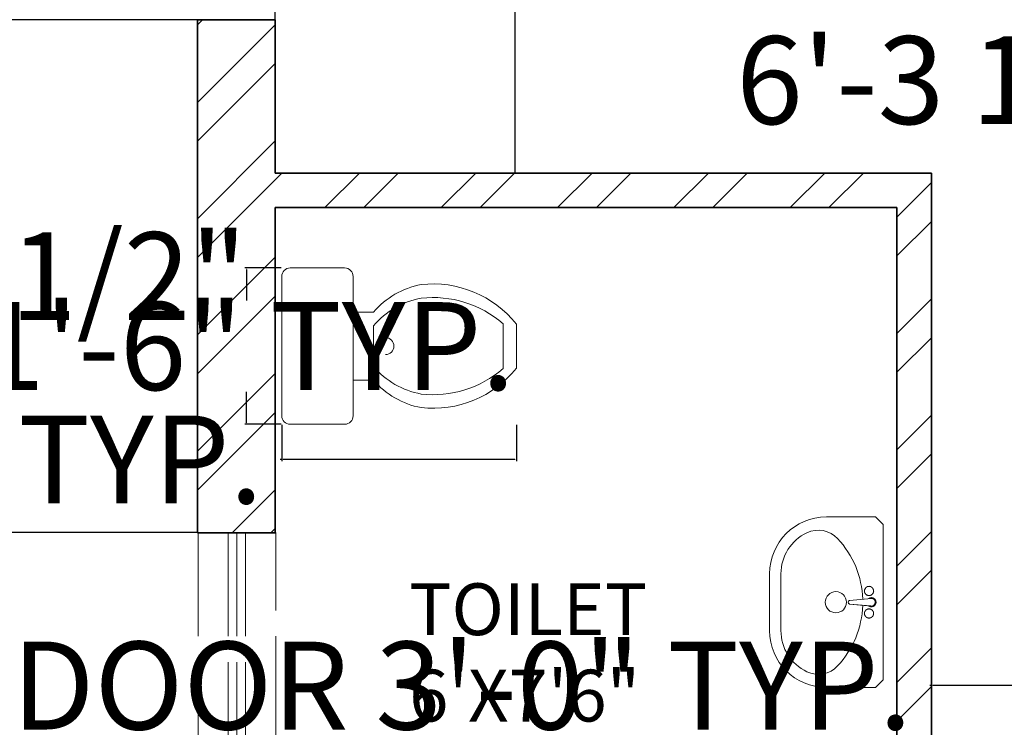
# Model space of a CAD drawing. Units: inches. Extents: x 1812 to 2791, y 2306 to 2959.
# Tile 3 of 8: x 1870 to 1984, y 2774 to 2856. Entities that reach past the tile are written whole.
import ezdxf

# ---------------------------------------------------------------- set-up
doc = ezdxf.new("R2010")
doc.units = ezdxf.units.IN
doc.linetypes.add('ACAD_ISO02W100', pattern=[15, 12, -3])
doc.layers.get('Defpoints').update_dxf_attribs({"lineweight": 50})
for name, color, linetype, lineweight in [('A-ANNO-DIMS', 2, 'Continuous', 18), ('A-AREA-IDEN', 7, 'Continuous', 18), ('A-FLOR-CASE', 8, 'Continuous', 18), ('A-FLOR-FIXT', 9, 'Continuous', 18), ('A-GLAZ-VENT', 6, 'ACAD_ISO02W100', 13), ('A-WALL-PATT', 8, 'Continuous', 13), ('WALL', 7, 'Continuous', 35)]:
    doc.layers.add(name, color=color, linetype=linetype, lineweight=lineweight)
doc.styles.get("Standard").update_dxf_attribs({"font": 'arial.ttf'})
doc.dimstyles.get("Standard").update_dxf_attribs({"dimtxt": 10.18, "dimasz": 0.18, "dimexe": 0.18, "dimexo": 0.0625, "dimgap": 0.09, "dimtad": 0, "dimtih": 1, "dimtoh": 1, "dimdec": 0, "dimzin": 0, "dimdsep": 46, "dimlunit": 3, "dimtxsty": 'Standard', "dimcen": 0.09, "dimadec": 0, "dimazin": 0, "dimtfac": 1, "dimtdec": 0, "dimtofl": 0, "dimtmove": 0, "dimatfit": 3, "dimfxl": 1, "dimtolj": 1, "dimtzin": 0, "dimarcsym": 0})

# ---------------------------------------------------------------- blocks, each defined once
blk = doc.blocks.new('A$C2AC94788')
for p, q in [((0.0250000842625013, 0.6899999873276103), (0.4350000842623559, 0.6899999873276103)), ((8.42619556e-08, 0.5049999873299384), (8.42619556e-08, 0.664999987326155)), ((0.4600000842619921, 0.664999987326155), (0.4600000842619921, 0.5049999873299384)), ((0.4350000842623559, 0.4799999873284833), (0.0250000842625013, 0.4799999873284833)), ((0.1300000842620648, 0.4799999873284833), (0.1300000842620648, 0.4199999873308116)), ((0.3300000842618829, 0.4199999873308116), (0.3300000842618829, 0.4799999873284833)), ((0.1700000842620284, 0.4199999873308116), (0.2900000842619192, 0.4199999873308116)), ((0.1640625266463758, 0.0391832446184708), (0.2959376418775719, 0.0391832446184708)), ((0.2290625266468851, 0.0391832446184708), (0.2300046331329213, 0.0391832446184708)), ((0.2309376418770626, 0.0391832446184708), (0.2299955353910263, 0.0391832446184708)), ((0.1650000842619192, -1.26747182e-08), (0.2950000842620284, -1.26747182e-08))]:
    blk.add_line(p, q)
for centre, radius, start, end in [((0.0250000842625013, 0.664999987326155), 0.025, 90, 180), ((0.4350000842623559, 0.664999987326155), 0.025, 0, 90), ((0.0250000842625013, 0.5049999873299384), 0.025, 180, 270), ((0.4350000842623559, 0.5049999873299384), 0.025, 270, 0), ((0.2874442183401697, 0.2355819240110577), 0.2424843859558644, 130.488541879527, 169.445013547103), ((0.3274442183401334, 0.2355819240110577), 0.2424843859558644, 130.488541879527, 169.445013547103), ((0.1325559501838143, 0.2355819240110577), 0.2424843859558745, 10.55498645289699, 49.51145812047296), ((0.1725559501837779, 0.2355819240110577), 0.2424843859558745, 10.55498645289699, 49.51145812047296), ((0.2300000842624286, 0.3849999873273191), 0.025, 180, 0), ((0.3600593119572294, 0.2447691737834247), 0.3129857136460789, 173.5368801771597, 231.4482773914608), ((0.4000593119571932, 0.2447691737834248), 0.3129857136460972, 173.5368801771598, 221.0603827222079), ((0.0999408565667182, 0.2447691737834248), 0.3129857136460789, 308.5517226085392, 6.463119822840183), ((0.0599408565667545, 0.2447691737834248), 0.3129857136460896, 318.9396172777922, 6.463119822840183)]:
    blk.add_arc(centre, radius, start, end)
blk = doc.blocks.new('s_46')
at = {"ltscale": 600}
h = blk.add_hatch(color=256, dxfattribs=at)
edge = h.paths.add_edge_path()
edge.add_line((13.45184378023259, 62.04360352296498), (14.15927104179718, 54.09782096462731))
edge.add_ellipse((4.212458010588306, 52.31250418393756), major_axis=(-10.10576298371302, 2.5e-15), ratio=1, start_angle=540, end_angle=550.1754626554052, ccw=False)
edge.add_arc((4.212458010588306, 52.31250418393756), 10.10576298371302, 270, 360, ccw=False)
edge.add_line((4.212458010588306, 42.20674120020703), (4.212458010588306, 41.28018079043977))
edge.add_line((4.212458010588306, 41.28018079040339), (11.85106942148559, 41.28018079040339))
edge.add_arc((4.212458010588306, 52.31250418393756), 13.41866400745597, 664.6981342835142, 766.4847699121552)
h.paths.add_polyline_path([(4.212458010588306, 41.28018079040339), (-3.426153400272596, 41.28018079040339, 0.152566653256377), (4.212458010588306, 38.8938401764608)])
h.paths.add_polyline_path([(11.85106942144921, 41.28018079040339), (4.212458010588306, 41.28018079040339), (4.212458010588306, 38.8938401764608, 0.1525666532563772)])
h.paths.add_polyline_path([(-5.734355020395014, 54.09782096461277), (-5.026927758881356, 62.04360352296498, 0.4758332592079194), (-3.426153400272596, 41.28018079040339), (4.212458010588306, 41.28018079040339), (4.212458010588306, 42.20674120020703, -0.4672400657637396)])
for p, q in [((-5.893304973142221, 52.31250418385025), (-0.714987907151226, 110.4750654234667)), ((-5.893304973142221, 52.31250418385025), (-0.714987907151226, 110.4750654234667)), ((9.139903928502463, 110.475065423554), (14.15927104174625, 54.09782096461277)), ((14.31822099431883, 52.31250418385025), (9.139903928502463, 110.475065423554)), ((14.15927104174625, 54.09782096461277), (14.31822099431883, 52.31250418385025))]:
    blk.add_line(p, q, dxfattribs=at)
blk.add_lwpolyline([(-220.7875419894117, 171.2801807903452, -0.4142135623730951), (-70.7875419894117, 321.2801807903452), (79.2124580105883, 321.2801807904325, -0.4142135623730951), (229.2124580105883, 171.2801807904325), (229.2124580105883, 41.28018079040339), (209.2124580107047, 21.2801807904325), (-200.7875419893535, 21.28018079034518), (-220.7875419894117, 41.28018079040339)], format="xyb", close=True, dxfattribs=at)
blk.add_lwpolyline([(12.26164246437838, 75.41187665969483, 0.1816379869150311), (172.1859176590806, 141.5383421540609, 0.3263505073803008), (187.6570333366981, 222.6589125997853, 0.2898144196813102), (79.21245801076293, 291.2801807904325), (-70.78754198923707, 291.2801807903452, 0.2898144196813102), (-179.2321173155214, 222.658912599698, 0.3263505073803008), (-163.7610016377293, 141.5383421540609, 0.1816379869150315), (-3.836726442852523, 75.41187665960751)], format="xyb", dxfattribs=at)
for points in [[(-16.83803374727722, 67.43055756771354), (-17.02338931558188, 67.50428807432763), (-17.22058725368697, 67.56961317334208), (-17.42189012444578, 67.6347039079701), (-17.61956049106084, 67.70773132116301), (-17.80586091603618, 67.79686645595939), (-17.97305396257434, 67.91028035557245), (-18.11578784312587, 68.05326030802098), (-18.23825336818117, 68.21955858168076), (-18.34702699835179, 68.40004368982045), (-18.44868519355077, 68.58558414605795), (-18.54980441438965, 68.76704846357461), (-18.65696112113073, 68.9353051558137), (-18.77673177386168, 69.08122273621848), (-18.91569283319404, 69.19566971814493), (-19.07841429975815, 69.27267628890695), (-19.26144033775199, 69.31891933156292), (-19.45930865121772, 69.34423740339116), (-19.66655694507062, 69.35846906132065), (-19.87772292352747, 69.37145286262967), (-20.08734429115429, 69.39302736415993), (-20.2899587523425, 69.43303112310241), (-20.48010401183274, 69.50130269664805), (-20.65391131333308, 69.60429419830325), (-20.81388605764368, 69.73491196823306), (-20.96412718523061, 69.8826759030926), (-21.10873363655992, 70.03710589953698), (-21.25180435174844, 70.18772185422131), (-21.39743827126222, 70.3240436638007), (-21.54973433539272, 70.43559122501756), (-21.71279148443137, 70.5118844343524), (-21.88955151231494, 70.54600451889564), (-22.07832762773614, 70.54527802669325), (-22.27627589285839, 70.52059283622657), (-22.4805523698451, 70.48283682571491), (-22.68831312085968, 70.44289787355228), (-22.89671420806553, 70.41166385821998), (-23.10291169380071, 70.40002265802468), (-23.30406164005399, 70.41886215136037), (-23.49802141042892, 70.4753938675276), (-23.68545357254334, 70.56212393892929), (-23.86772199510597, 70.66788214896224), (-24.04619054717477, 70.78149828102323), (-24.22222309763311, 70.89180211850908), (-24.39718351518968, 70.98762344472925), (-24.57243566872785, 71.05779204316786), (-24.74934342730558, 71.09113769704709), (-24.92903553397628, 71.08022740500746), (-25.11170022917213, 71.03257702605333), (-25.2972906283685, 70.95943963443278), (-25.48575984616764, 70.8720683044812), (-25.67706099752104, 70.7817161102721), (-25.87114719772944, 70.69963612605352), (-26.0679715613951, 70.63708142607356), (-26.26748720381875, 70.60530508466763), (-26.46941223740578, 70.61182491958607), (-26.67252476507565, 70.64921772302478), (-26.87536788737634, 70.70632503094384), (-27.07648470485583, 70.77198837930337), (-27.27441831788747, 70.8350493038015), (-27.46771182701923, 70.88434934031102), (-27.6549083327991, 70.90873002487933), (-27.83455093560042, 70.8970328932919), (-28.00620139669627, 70.84190539614065), (-28.17349611973623, 70.75121864315588), (-28.34109016874572, 70.63664965887438), (-28.51363860827405, 70.50987546765828), (-28.69579650234664, 70.38257309404435), (-28.89221891516354, 70.26641956248204), (-29.10756091127405, 70.17309189750813), (-29.3464775547036, 70.11426712348475), (-29.61160253512208, 70.0940409177856), (-29.89748404390411, 70.0861835690448), (-30.19664889771957, 70.05688401864609), (-30.50162391323829, 69.9723312081478), (-30.80493590747938, 69.79871407902101), (-31.09911169676343, 69.50222157256212), (-31.37667809793493, 69.0490426304168), (-31.63016192783834, 68.40536619405611), (-32.32050594605971, 68.4500712644367), (-32.84873653826071, 68.3918758847285), (-33.24226493795868, 68.25193804170704), (-33.52850237919483, 68.0514157223224), (-33.73486009566113, 67.8114669136994), (-33.88874932087492, 67.5532496026135), (-34.01758128887741, 67.29792177610216), (-34.14876723336056, 67.06664142102818), (-34.30371923936764, 66.87550954936887), (-34.47985279804561, 66.72039927294827), (-34.66858425136889, 66.59212672835565), (-34.86132994201034, 66.48150805244222), (-35.04950621211901, 66.37935938188457), (-35.22452940384392, 66.27649685335928), (-35.37781585985795, 66.16373660371755), (-35.50078192248475, 66.03189476963598), (-35.58785390376579, 65.87432967920904), (-35.64549799636007, 65.69456842611542), (-35.68319036299363, 65.49868029527715), (-35.7104071660433, 65.2927345718781), (-35.73662456823513, 65.08280054092756), (-35.77131873212056, 64.87494748734753), (-35.82396582007641, 64.67524469623459), (-35.90404199482873, 64.48976145259803), (-36.01774371694773, 64.3227640100813), (-36.15814863995183, 64.17130649695173), (-36.31505471485434, 64.0306400101108), (-36.47825989319244, 63.89601564637269), (-36.63756212632871, 63.76268450255157), (-36.78275936545106, 63.62589767554891), (-36.90364956192207, 63.48090626226621), (-36.99003066710429, 63.32296135951764), (-37.03518227743916, 63.14869254492805), (-37.04631056915969, 62.96024331927765), (-37.03410336375237, 62.7611356638954), (-37.00924848217983, 62.55489156045951), (-36.98243374592858, 62.34503299021162), (-36.96434697631048, 62.13508193491725), (-36.96567599463743, 61.92856037581805), (-36.99710862222128, 61.72899029450491), (-37.06570762058254, 61.53896291530691), (-37.16403551277472, 61.35734643402975), (-37.28102976223454, 61.18207828939194), (-37.40562783187488, 61.0110959201993), (-37.52676718513249, 60.84233676508302), (-37.63338528544409, 60.67373826284892), (-37.7144195958972, 60.50323785204091), (-37.75880757992855, 60.32877297155209), (-37.75920177751686, 60.14875038337777), (-37.72311503690435, 59.96345414296957), (-37.66177528270055, 59.77363762940512), (-37.58641044021351, 59.58005422132555), (-37.5082484340528, 59.38345729780849), (-37.43851718935184, 59.18460023758234), (-37.38844463089481, 58.98423641963745), (-37.36925868364051, 58.78311922278953), (-37.38844463089481, 58.58200202594161), (-37.43851718935184, 58.38163820799673), (-37.5082484340528, 58.18278114777058), (-37.58641044021351, 57.98618422425352), (-37.66177528287517, 57.79260081626126), (-37.72311503690435, 57.6027843026095), (-37.75920177751686, 57.4174880622013), (-37.75880757992855, 57.23746547402697), (-37.7144195958972, 57.06300059353816), (-37.63338528544409, 56.89250018273014), (-37.52676718530711, 56.72390168049606), (-37.40562783187488, 56.55514252537978), (-37.28102976223454, 56.38416015618713), (-37.16403551277472, 56.20889201154932), (-37.06570762058254, 56.02727553035947), (-36.99710862222128, 55.83724815107416), (-36.96567599463743, 55.63767806976102), (-36.96434697631048, 55.43115651066182), (-36.98243374592858, 55.22120545536745), (-37.00924848217983, 55.01134688520687), (-37.03410336375237, 54.80510278168367), (-37.04631056933431, 54.60599512638873), (-37.03518227743916, 54.41754590065102), (-36.99003066710429, 54.24327708606142), (-36.90364956192207, 54.08533218331285), (-36.78275936545106, 53.94034077003016), (-36.63756212632871, 53.80355394302751), (-36.47825989319244, 53.67022279920639), (-36.31505471502896, 53.53559843546827), (-36.15814863995183, 53.39493194862734), (-36.01774371712236, 53.24347443549777), (-35.90404199482873, 53.07647699298104), (-35.82396582007641, 52.89099374934449), (-35.77131873212056, 52.69129095823155), (-35.73662456823513, 52.48343790465151), (-35.71040716621792, 52.27350387370098), (-35.68319036299363, 52.06755815021461), (-35.64549799653469, 51.87167001946363), (-35.58785390376579, 51.69190876637003), (-35.50078192248475, 51.53434367594309), (-35.3778353385278, 51.40284301002975), (-35.22468523163116, 51.29247093791491), (-35.05003213009331, 51.19609060572111), (-34.86257656256203, 51.10656515930895), (-34.67101905716118, 51.01675774488831), (-34.48406014236389, 50.91953150840708), (-34.31040034646867, 50.80774959607516), (-34.15874019777402, 50.67427515375311), (-34.03505195630714, 50.51453334218241), (-33.93439480883535, 50.3341973797942), (-33.84909967368003, 50.14150249981321), (-33.77149746881332, 49.94468393520219), (-33.69391911290586, 49.75197691909852), (-33.60869552427903, 49.57161668455228), (-33.50815762107959, 49.41183846470085), (-33.38463632145431, 49.28087749250699), (-33.23284944484476, 49.18408373402781), (-33.05706241185544, 49.11526608630083), (-32.86392754490953, 49.06534817945794), (-32.66009716555709, 49.02525364354369), (-32.45222359569743, 48.98590610860265), (-32.24695915722987, 48.93822920459206), (-32.05095617187908, 48.87314656155649), (-31.870866961719, 48.78158180962782), (-31.71133844077122, 48.65761859554914), (-31.5689958925941, 48.50798063381808), (-31.43845919286832, 48.34255165536887), (-31.31434821744915, 48.17121539139771), (-31.19128284219187, 48.00385557310073), (-31.06388294277713, 47.85035593167413), (-30.92676839523483, 47.72060019822674), (-30.77455907507101, 47.62447210386745), (-30.60346923320321, 47.56846716045401), (-30.41609062027419, 47.54552800310193), (-30.21660936163971, 47.54520904741366), (-30.00921158283018, 47.55706470907898), (-29.79808340937598, 47.570649403875), (-29.58741096680751, 47.57551754757878), (-29.38138038065517, 47.56122355579281), (-29.18417777627474, 47.51732184420689), (-28.99883273948217, 47.43692629240103), (-28.8237486963626, 47.32738863455597), (-28.65617253311211, 47.19962006882997), (-28.49335113610141, 47.06453179311938), (-28.33253139152657, 46.9330350055825), (-28.1709601857583, 46.81604090429027), (-28.00588440499268, 46.72446068713907), (-27.83455093577504, 46.66920555219985), (-27.6549083327991, 46.65750842061243), (-27.46771182701923, 46.68188910518074), (-27.27441831788747, 46.73118914177758), (-27.07648470485583, 46.7942500662757), (-26.87536788755096, 46.85991341454792), (-26.67252476525027, 46.91702072246698), (-26.4694122375804, 46.95441352590569), (-26.26748720399337, 46.96093336082412), (-26.06797156156972, 46.9291570194182), (-25.87114719772944, 46.86660231943824), (-25.67706099769566, 46.78452233530697), (-25.48575984616764, 46.69417014101054), (-25.2972906283685, 46.60679881105898), (-25.11170022934675, 46.53366141943843), (-24.92903553397628, 46.4860110404843), (-24.74934342730558, 46.47510074844467), (-24.57243566890247, 46.50844640232389), (-24.39718351536431, 46.57861500076251), (-24.22222309780773, 46.67443632698268), (-24.0461905473494, 46.78474016446853), (-23.86772199528059, 46.89835629652953), (-23.68545357254334, 47.00411450656247), (-23.49802141060354, 47.09084457796416), (-23.30406164022861, 47.14737629413138), (-23.10291169380071, 47.16621578746708), (-22.89671420806553, 47.15457458727178), (-22.68831312085968, 47.12334057193948), (-22.4805523698451, 47.08340161977685), (-22.27627589285839, 47.04564560926519), (-22.07832762791077, 47.02096041871118), (-21.88955151248956, 47.02023392650881), (-21.71279148443137, 47.05435401113937), (-21.54973433539272, 47.1306472204742), (-21.39743827126222, 47.24219478160375), (-21.25180435174844, 47.37851659118314), (-21.10873363655992, 47.52913254586746), (-20.96412718540523, 47.68356254231185), (-20.81388605764368, 47.83132647717138), (-20.65391131333308, 47.9619442471012), (-20.48010401200736, 48.0649357488437), (-20.28995875251712, 48.13320732230204), (-20.08734429115429, 48.17321108133183), (-19.87772292352747, 48.1947855828621), (-19.66655694507062, 48.2077693840838), (-19.45930865139235, 48.2220010421006), (-19.26144033775199, 48.24731911384152), (-19.07841429993277, 48.29356215667212), (-18.91569283319404, 48.37056872743414), (-18.77673177403631, 48.48501570936059), (-18.65696112113073, 48.63093328976538), (-18.54980441456428, 48.79918998200446), (-18.44868519372539, 48.98065429960843), (-18.34702699835179, 49.16619475575862), (-18.2382533683558, 49.34667986398562), (-18.11578784312587, 49.5129781376454), (-17.97305396274896, 49.6559580900066), (-17.8058609162108, 49.76937198961969), (-17.61956049106084, 49.85850712450337), (-17.4218901246204, 49.93153453769628), (-17.22058725368697, 49.996625272237), (-17.02338931558188, 50.06195037133875), (-16.83803374727722, 50.13568087795284), (-16.67225798609434, 50.22598783511785), (-16.53379946883069, 50.34104228604701), (-16.42766593385022, 50.48645191569812), (-16.34794632298872, 50.65757097714231), (-16.28599987912457, 50.84719036528259), (-16.23318584513618, 51.04810097528389), (-16.18086346407654, 51.25309370196191), (-16.12039197882404, 51.45495944039431), (-16.04313063243171, 51.64648908557137), (-15.94043866742868, 51.82047353248345), (-15.8067031877581, 51.97190354572376), (-15.64842273970134, 52.10456936812261), (-15.47512373042991, 52.22446111202589), (-15.29633256676607, 52.33756888969219), (-15.12157565605594, 52.44988281364204), (-14.96037940529641, 52.567392996134), (-14.82227022130973, 52.69608954960131), (-14.71677451161667, 52.84196258638985), (-14.6501372611965, 53.00919824198354), (-14.61547776852967, 53.19476674450561), (-14.60263391025364, 53.3938343450427), (-14.60144356318051, 53.60156729485606), (-14.60174460412236, 53.81313184503233), (-14.59337490954203, 54.02369424700736), (-14.566172356077, 54.22842075169319), (-14.50997482053935, 54.42247761052567), (-14.41809999983525, 54.6024088327249), (-14.29778487142175, 54.77026946117985), (-14.1597462335485, 54.92949229647638), (-14.01470088359201, 55.08351013963693), (-13.87336561962729, 55.23575579150929), (-13.7464572393801, 55.38966205302859), (-13.64469254092546, 55.54866172495531), (-13.5787883218145, 55.71618760822457), (-13.55583441938506, 55.89474125843844), (-13.56841282837558, 56.08309925056528), (-13.60547858278733, 56.27910691397847), (-13.65598671662155, 56.48060957840062), (-13.70889226370491, 56.68545257346704), (-13.7531502583879, 56.89148122872575), (-13.7777157346718, 57.09654087381204), (-13.77154372638324, 57.29847683827393), (-13.72730239736847, 57.49560352915432), (-13.65251243085367, 57.68811166286468), (-13.55840763938613, 57.8766610333987), (-13.45622183586238, 58.06191143448813), (-13.35718883317895, 58.24452266012667), (-13.27254244388314, 58.42515450413339), (-13.2135164810461, 58.60446676041465), (-13.19134475721512, 58.78311922278953), (-13.2135164810461, 58.96177168516442), (-13.27254244388314, 59.14108394144569), (-13.35718883317895, 59.3217157854524), (-13.45622183586238, 59.50432701109093), (-13.55840763938613, 59.68957741218037), (-13.65251243085367, 59.87812678271438), (-13.72730239736847, 60.07063491642475), (-13.77154372638324, 60.26776160730515), (-13.7777157346718, 60.46969757176703), (-13.7531502583879, 60.67475721685332), (-13.70889226370491, 60.88078587211203), (-13.65598671662155, 61.08562886717845), (-13.60547858278733, 61.2871315316006), (-13.56841282837558, 61.48313919501379), (-13.55583441938506, 61.67149718714063), (-13.5787883218145, 61.8500508373545), (-13.64469254092546, 62.01757672062377), (-13.7464572393801, 62.17657639255048), (-13.87336561962729, 62.33048265406978), (-14.01470088359201, 62.48272830594214), (-14.15974623337388, 62.63674614910269), (-14.29778487142175, 62.79596898448653), (-14.41809999983525, 62.96382961285416), (-14.50997482053935, 63.14376083514071), (-14.566172356077, 63.33781769388588), (-14.59337490936741, 63.5425441985717), (-14.60174460412236, 63.75310660054674), (-14.60144356318051, 63.96467115081032), (-14.60263391025364, 64.17240410053635), (-14.61547776835505, 64.37147170116077), (-14.65013726102188, 64.55704020359553), (-14.71677451144205, 64.7242758591892), (-14.82227022130973, 64.87014889597776), (-14.96037940529641, 64.99884544944507), (-15.12157565605594, 65.11635563193704), (-15.29633256676607, 65.22866955588688), (-15.47512373042991, 65.3417773336405), (-15.64842273970134, 65.46166907745646), (-15.8067031877581, 65.59433489985531), (-15.94043866742868, 65.74576491309563), (-16.04313063225709, 65.9197493600077), (-16.12039197882404, 66.11127900527208), (-16.18086346407654, 66.31314474370447), (-16.23318584513618, 66.5181374703825), (-16.28599987912457, 66.71904808029649), (-16.34794632298872, 66.90866746843676), (-16.42766593385022, 67.07978652988095), (-16.53379946883069, 67.22519615953206), (-16.67225798609434, 67.34025061046123)], [(22.08090273779817, 61.08562886709115), (22.03039460413856, 61.2871315315133), (21.99332884972682, 61.48313919501379), (21.9807504407363, 61.67149718705331), (22.00370434316574, 61.85005083726719), (22.06960856210208, 62.01757672053645), (22.17137326073134, 62.17657639246318), (22.29828164080391, 62.33048265398247), (22.43961690476863, 62.48272830585483), (22.58466225472512, 62.63674614901538), (22.72270089277299, 62.79596898439923), (22.84301602118649, 62.96382961276686), (22.93489084189059, 63.1437608350534), (22.99108837742824, 63.33781769379857), (23.01829093071865, 63.5425441985717), (23.0266606254736, 63.75310660045943), (23.02635958453175, 63.96467115072301), (23.02754993160488, 64.17240410053635), (23.04039378970629, 64.37147170107346), (23.07505328237312, 64.55704020350822), (23.14169053279329, 64.72427585910191), (23.24718624266097, 64.87014889589045), (23.38529542664764, 64.99884544935776), (23.54649167740717, 65.11635563193704), (23.7212485881173, 65.22866955579956), (23.90003975178115, 65.34177733355318), (24.07333876105258, 65.46166907736915), (24.23161920910934, 65.594334899768), (24.36535468877992, 65.74576491300832), (24.46804665360833, 65.9197493600077), (24.54530800017528, 66.11127900518477), (24.60577948542777, 66.31314474361714), (24.65810186648742, 66.51813747029519), (24.71091590047581, 66.71904808020918), (24.77286234433996, 66.90866746834945), (24.85258195520146, 67.07978652979364), (24.95871549018193, 67.22519615953206), (25.09717400744558, 67.34025061046123), (25.26294976862846, 67.43055756771354), (25.44830533693312, 67.50428807432763), (25.64550327503821, 67.56961317334208), (25.84680614579702, 67.6347039079701), (26.04447651241208, 67.70773132116301), (26.23077693756204, 67.79686645595939), (26.3979699841002, 67.91028035557245), (26.54070386447711, 68.05326030802098), (26.66316938970704, 68.21955858168076), (26.77194301970303, 68.40004368982045), (26.87360121507663, 68.58558414605795), (26.97472043591552, 68.76704846357461), (27.08187714248197, 68.9353051558137), (27.20164779538754, 69.08122273621848), (27.34060885454528, 69.19566971814493), (27.50333032128401, 69.27267628890695), (27.68635635910323, 69.31891933165025), (27.88422467274358, 69.34423740347847), (28.09147296642186, 69.35846906140794), (28.30263894487871, 69.37145286262967), (28.51226031250553, 69.39302736424725), (28.71487477386836, 69.43303112318972), (28.90502003318398, 69.50130269673537), (29.07882733468432, 69.60429419839056), (29.23880207899492, 69.73491196832038), (29.38904320658185, 69.88267590317992), (29.53364965791116, 70.0371058996243), (29.67672037309967, 70.18772185430862), (29.82235429261346, 70.324043663888), (29.97465035674395, 70.43559122501756), (30.1377075057826, 70.51188443443971), (30.31446753366618, 70.54600451898295), (30.50324364908738, 70.54527802678058), (30.70119191420963, 70.52059283622657), (30.90546839119634, 70.48283682571491), (31.11322914221091, 70.4428978736396), (31.32163022941677, 70.41166385830729), (31.52782771515195, 70.400022658112), (31.72897766157985, 70.41886215144768), (31.92293743178016, 70.4753938675276), (32.11036959389458, 70.56212393892929), (32.29263801663183, 70.66788214896224), (32.47110656870063, 70.78149828102323), (32.64713911898434, 70.89180211850908), (32.82209953654092, 70.98762344481656), (32.99735169025371, 71.05779204316786), (33.17425944865681, 71.09113769704709), (33.35395155532751, 71.08022740500746), (33.53661625069799, 71.03257702605333), (33.72220664971974, 70.9594396345201), (33.91067586751888, 70.8720683044812), (34.1019770190469, 70.7817161102721), (34.29606321908068, 70.69963612605352), (34.49288758292096, 70.63708142616088), (34.69240322534461, 70.60530508466763), (34.89432825893164, 70.61182491958607), (35.09744078660151, 70.64921772302478), (35.3002839089022, 70.70632503103116), (35.50140072620707, 70.77198837930337), (35.6993343392387, 70.8350493038015), (35.89262784837047, 70.88434934039833), (36.07982435415034, 70.90873002487933), (36.25946695695166, 70.8970328932919), (36.43111741804751, 70.84190539614065), (36.59841214108747, 70.75121864315588), (36.76600619009696, 70.63664965887438), (36.93855462962529, 70.50987546765828), (37.12071252369788, 70.38257309404435), (37.3171349366894, 70.26641956248204), (37.53247693262529, 70.17309189750813), (37.77139357605483, 70.11426712348475), (38.03651855647331, 70.0940409177856), (38.32240006525535, 70.0861835690448), (38.62156491907081, 70.05688401864609), (38.92653993476415, 69.9723312081478), (39.22985192883061, 69.79871407893368), (39.52402771811467, 69.50222157256212), (39.80159411928616, 69.0490426304168), (40.05507794918957, 68.4053661939688), (40.74542196741094, 68.4500712644367), (41.27365255961194, 68.3918758846412), (41.66718095948453, 68.25193804161972), (41.95341840054607, 68.0514157223224), (42.15977611701236, 67.8114669136121), (42.31366534240078, 67.5532496025262), (42.44249731022864, 67.29792177601485), (42.57368325471179, 67.06664142094087), (42.72863526071887, 66.87550954936887), (42.90476881939684, 66.72039927286096), (43.09350027272012, 66.59212672826834), (43.28624596336157, 66.48150805235491), (43.47442223347025, 66.37935938179726), (43.64944542536977, 66.27649685335928), (43.80273188138381, 66.16373660371755), (43.92569794383598, 66.03189476963598), (44.01276992511703, 65.87432967912173), (44.0704140177113, 65.69456842602813), (44.10810638434486, 65.49868029527715), (44.13532318739453, 65.2927345718781), (44.16154058958636, 65.08280054084025), (44.19623475347179, 64.87494748726021), (44.24888184142765, 64.67524469614727), (44.32895801617997, 64.48976145251072), (44.44265973829897, 64.32276400999397), (44.58306466130307, 64.17130649695173), (44.73997073620558, 64.03064001002348), (44.90317591454368, 63.89601564628538), (45.06247814767994, 63.76268450246425), (45.20767538680229, 63.6258976754616), (45.3285655832733, 63.4809062621789), (45.41494668845553, 63.32296135943034), (45.46009829879039, 63.14869254484074), (45.47122659051092, 62.96024331919034), (45.45901938492898, 62.76113566380809), (45.43416450353106, 62.5548915603722), (45.40734976727981, 62.34503299021162), (45.38926299766171, 62.13508193482994), (45.39059201598866, 61.92856037573074), (45.42202464357251, 61.7289902944176), (45.49062364193377, 61.53896291521959), (45.58895153412595, 61.35734643394243), (45.70594578341115, 61.18207828939194), (45.83054385322611, 61.01109592011198), (45.95168320648371, 60.84233676508302), (46.05830130679533, 60.67373826276162), (46.13933561724843, 60.50323785204091), (46.18372360127978, 60.32877297146479), (46.1841177988681, 60.14875038329046), (46.14803105825558, 59.96345414296957), (46.08669130405178, 59.77363762931782), (46.01132646156474, 59.58005422123824), (45.93316445540404, 59.38345729772118), (45.86343321070308, 59.18460023749503), (45.81336065224604, 58.98423641955014), (45.79417470499175, 58.78311922270222), (45.81336065224604, 58.58200202585431), (45.86343321070308, 58.38163820790942), (45.93316445540404, 58.18278114777058), (46.01132646156474, 57.98618422416621), (46.08669130405178, 57.79260081617394), (46.14803105808095, 57.6027843025222), (46.1841177988681, 57.4174880622013), (46.18372360127978, 57.23746547393966), (46.13933561724843, 57.06300059345085), (46.05830130679533, 56.89250018273014), (45.95168320648371, 56.72390168040874), (45.83054385322611, 56.55514252529247), (45.70594578341115, 56.38416015609982), (45.58895153412595, 56.20889201154932), (45.49062364193377, 56.02727553027216), (45.42202464339789, 55.83724815107416), (45.39059201598866, 55.63767806976102), (45.38926299766171, 55.43115651066182), (45.40734976727981, 55.22120545528014), (45.43416450335644, 55.01134688511957), (45.45901938492898, 54.80510278159636), (45.47122659051092, 54.60599512630142), (45.46009829879039, 54.41754590056371), (45.41494668845553, 54.24327708597411), (45.32856558309868, 54.08533218322554), (45.20767538662767, 53.94034076994285), (45.06247814750532, 53.8035539429402), (44.90317591454368, 53.67022279920639), (44.73997073620558, 53.53559843538096), (44.58306466130307, 53.39493194854004), (44.44265973829897, 53.24347443541046), (44.32895801617997, 53.07647699298104), (44.24888184125302, 52.89099374934449), (44.19623475329717, 52.69129095823155), (44.16154058958636, 52.48343790465151), (44.13532318739453, 52.27350387361366), (44.10810638434486, 52.06755815021461), (44.0704140177113, 51.87167001946363), (44.01276992511703, 51.69190876628272), (43.92569794366136, 51.53434367585578), (43.80275135970442, 51.40284301002975), (43.64960125280776, 51.29247093791491), (43.47494815144455, 51.1960906056338), (43.28749258373863, 51.10656515922165), (43.09593507851241, 51.01675774480099), (42.90897616371512, 50.91953150840708), (42.73531636764528, 50.80774959598784), (42.58365621895063, 50.67427515375311), (42.45996797765838, 50.51453334218241), (42.35931083018658, 50.3341973797942), (42.27401569485664, 50.14150249981321), (42.19641349016455, 49.94468393520219), (42.1188351342571, 49.75197691909852), (42.03361154545564, 49.57161668455228), (41.9330736422562, 49.41183846461354), (41.80955234280554, 49.28087749250699), (41.65776546602137, 49.1840837339405), (41.48197843320668, 49.11526608630083), (41.28884356608614, 49.06534817945794), (41.0850131867337, 49.02525364354369), (40.87713961687405, 48.98590610851534), (40.67187517840648, 48.93822920459206), (40.47587219323031, 48.87314656155649), (40.29578298289561, 48.78158180962782), (40.13625446194782, 48.65761859554914), (39.99391191377072, 48.50798063373076), (39.86337521404493, 48.34255165528157), (39.73926423862577, 48.17121539139771), (39.61619886336848, 48.00385557310073), (39.48879896395374, 47.85035593167413), (39.35168441641144, 47.72060019813944), (39.19947509624762, 47.62447210378013), (39.02838525455445, 47.56846716045401), (38.8410066414508, 47.54552800310193), (38.64152538281633, 47.54520904732635), (38.43412760400679, 47.55706470907898), (38.22299943072721, 47.570649403875), (38.01232698798413, 47.57551754757878), (37.80629640183179, 47.56122355579281), (37.60909379745135, 47.51732184420689), (37.42374876065878, 47.43692629240103), (37.24866471753922, 47.32738863455597), (37.08108855428873, 47.19962006882997), (36.91826715727803, 47.06453179311938), (36.75744741270319, 46.9330350056698), (36.59587620693492, 46.81604090429027), (36.4308004261693, 46.72446068713907), (36.25946695695166, 46.66920555228716), (36.07982435397571, 46.65750842061243), (35.89262784837047, 46.68188910518074), (35.6993343392387, 46.73118914177758), (35.50140072620707, 46.7942500662757), (35.30028390872758, 46.85991341454792), (35.09744078642689, 46.91702072246698), (34.89432825875701, 46.954413525993), (34.69240322516998, 46.96093336082412), (34.49288758274633, 46.9291570194182), (34.29606321908068, 46.86660231943824), (34.10197701887228, 46.78452233530697), (33.91067586734425, 46.69417014109785), (33.72220664971974, 46.60679881105898), (33.53661625052337, 46.53366141943843), (33.35395155515289, 46.4860110404843), (33.17425944865681, 46.47510074844467), (32.99735169007909, 46.5084464024112), (32.82209953654092, 46.57861500076251), (32.64713911898434, 46.67443632707), (32.47110656852601, 46.78474016446853), (32.2926380164572, 46.89835629661684), (32.11036959389458, 47.00411450664979), (31.92293743178016, 47.09084457805147), (31.72897766140522, 47.14737629413138), (31.52782771497732, 47.16621578746708), (31.32163022941677, 47.15457458727178), (31.11322914203629, 47.12334057193948), (30.90546839102171, 47.08340161986416), (30.70119191420963, 47.0456456093525), (30.50324364908738, 47.02096041879849), (30.31446753366618, 47.02023392659611), (30.1377075057826, 47.05435401113937), (29.97465035674395, 47.13064722056151), (29.82235429261346, 47.24219478169106), (29.67672037309967, 47.37851659127045), (29.53364965791116, 47.52913254595478), (29.38904320658185, 47.68356254239916), (29.2388020788203, 47.8313264772587), (29.0788273345097, 47.96194424718851), (28.90502003318398, 48.06493574893102), (28.71487477369374, 48.13320732238935), (28.51226031250553, 48.17321108133183), (28.30263894487871, 48.19478558294941), (28.09147296642186, 48.20776938417111), (27.88422467256896, 48.22200104218791), (27.68635635892861, 48.24731911392882), (27.50333032110939, 48.29356215667212), (27.34060885454528, 48.37056872743414), (27.20164779521292, 48.48501570936059), (27.08187714248197, 48.63093328976538), (26.97472043574089, 48.79918998200446), (26.87360121490201, 48.98065429960843), (26.77194301952841, 49.16619475575862), (26.66316938953241, 49.34667986398562), (26.54070386447711, 49.51297813755809), (26.39796998392558, 49.6559580900066), (26.23077693738742, 49.76937198961969), (26.04447651223745, 49.85850712450337), (25.84680614579702, 49.93153453769628), (25.64550327486359, 49.996625272237), (25.44830533675849, 50.06195037133875), (25.26294976862846, 50.13568087795284), (25.09717400727095, 50.22598783520516), (24.95871549018193, 50.34104228604701), (24.85258195520146, 50.48645191561082), (24.77286234416534, 50.657570977055), (24.71091590030119, 50.84719036519527), (24.65810186648742, 51.04810097519657), (24.60577948542777, 51.2530937018746), (24.54530800017528, 51.45495944030699), (24.46804665360833, 51.64648908548406), (24.36535468877992, 51.82047353239614), (24.23161920910934, 51.97190354572376), (24.07333876105258, 52.1045693680353), (23.90003975160653, 52.22446111193858), (23.7212485881173, 52.33756888960488), (23.54649167740717, 52.44988281355472), (23.38529542647302, 52.56739299604669), (23.24718624266097, 52.696089549514), (23.14169053279329, 52.84196258630254), (23.07505328237312, 53.00919824189623), (23.04039378970629, 53.1947667444183), (23.02754993160488, 53.39383434495539), (23.02635958453175, 53.60156729476876), (23.02666062529898, 53.81313184503233), (23.01829093071865, 54.02369424692006), (22.99108837725362, 54.22842075169319), (22.93489084171597, 54.42247761043836), (22.84301602101186, 54.6024088327249), (22.72270089277299, 54.77026946109254), (22.58466225472512, 54.92949229638907), (22.43961690476863, 55.08351013963693), (22.29828164080391, 55.23575579150929), (22.17137326073134, 55.38966205294127), (22.06960856210208, 55.548661724868), (22.00370434316574, 55.71618760813726), (21.9807504407363, 55.89474125843844), (21.99332884972682, 56.08309925047797), (22.03039460413856, 56.27910691389115), (22.08090273779817, 56.48060957840062), (22.13380828505615, 56.68545257346704), (22.17806627973914, 56.89148122872575), (22.20263175602304, 57.09654087381204), (22.19645974773448, 57.29847683827393), (22.15221841871971, 57.49560352915432), (22.07742845220491, 57.68811166286468), (21.98332366073737, 57.87666103331139), (21.88113785721362, 58.06191143448813), (21.78210485453019, 58.24452266012667), (21.69745846523438, 58.42515450413339), (21.63843250239734, 58.60446676032734), (21.61626077856636, 58.78311922270222), (21.63843250239734, 58.96177168507711), (21.69745846523438, 59.14108394135837), (21.78210485453019, 59.32171578536508), (21.88113785721362, 59.50432701100362), (21.98332366073737, 59.68957741209306), (22.07742845220491, 59.87812678262708), (22.15221841871971, 60.07063491633743), (22.19645974773448, 60.26776160721784), (22.20263175602304, 60.46969757167971), (22.17806627973914, 60.67475721676601), (22.13380828505615, 60.88078587202471)]]:
    blk.add_lwpolyline(points, close=True, dxfattribs=at)
blk.add_circle((4.212458010588306, 146.2801807904034), 28, dxfattribs=at)
for centre, radius, start, end in [((4.212458010588306, 108.2109541267855), 5.422722861947412, 24.67830004152974, 155.3216999584702), ((4.212458010588306, 52.31250418393756), 10.10576298371233, 169.8245373479931, 0)]:
    blk.add_arc(centre, radius, start, end, dxfattribs=at)
for centre, major_axis, ratio, start_param, end_param in [((4.212458010762929, 110.475065423554), (-4.927445917859709, 1.2e-15), 0.6410240960233505, 3.141592653589793, 6.283185307179586), ((4.212458010588306, 52.31250418393756), (-10.10576298371302, 2.5e-15), 1, 6.105589980929039, 9.602373287019926)]:
    blk.add_ellipse(centre, major_axis=major_axis, ratio=ratio, start_param=start_param, end_param=end_param, dxfattribs=at)
blk = doc.blocks.new('VENT-24x9')
for p, q in [((3.499863851171994, 23.99973038050894), (3.499863851171994, -0.0002696194910641)), ((4.499863851171994, 23.99973038050894), (4.499863851171994, -0.0002696194910641)), ((5.499863851171994, 23.99973038050894), (5.499863851171994, -0.0002696194910641))]:
    blk.add_line(p, q)
blk.add_lwpolyline([(-0.0001361485951747, -0.0002696194910641), (8.999863851404825, -0.0002696194910641), (8.999863851171995, 23.99973038050894), (-0.0001361488280054, 23.99973038050894)], close=True)
blk = doc.blocks.new('*D42')
at = {"layer": 'A-ANNO-DIMS', "color": 0, "lineweight": -2, "transparency": 16777216}
for p, q in [((1975.370579728209, 2779.236987448721), (1975.190579728209, 2779.236987448721)), ((1975.370579728209, 2773.899487448718), (1975.370579728209, 2779.416987448721)), ((2011.190579728229, 2779.236987448721), (1975.550579728209, 2779.236987448721)), ((2011.370579728229, 2773.899487448718), (2011.370579728229, 2779.416987448721))]:
    blk.add_line(p, q, dxfattribs=at)
at = {"layer": 'A-ANNO-DIMS', "color": 0, "transparency": 16777216}
for points in [[(1975.550579728209, 2779.266987448721), (1975.550579728209, 2779.206987448721), (1975.370579728209, 2779.236987448721)], [(2011.190579728229, 2779.266987448721), (2011.190579728229, 2779.206987448721), (2011.370579728229, 2779.236987448721)]]:
    blk.add_solid(points, dxfattribs=at)
at = {"layer": 'Defpoints', "color": 0, "transparency": 16777216}
for p in [(1975.370579728209, 2779.236987448721), (1975.370579728209, 2773.836987448718), (2011.370579728229, 2773.836987448718)]:
    blk.add_point(p, dxfattribs=at)
at = {"layer": 'A-ANNO-DIMS', "color": 0, "transparency": 16777216, "insert": (1921.020197736394, 2779.236987448721), "char_height": 10.18, "attachment_point": 5}
blk.add_mtext('\\A1;DOOR 3\'-0" TYP.', dxfattribs=at)
blk = doc.blocks.new('*D51')
at = {"layer": 'A-ANNO-DIMS', "color": 0, "lineweight": -2, "transparency": 16777216}
for p, q in [((2010.613726114925, 2887.157800411407), (1995.646226114926, 2887.157800411407)), ((1995.826226114926, 2886.977800411407), (1995.826226114926, 2854.714874081257)), ((1995.826226114926, 2811.737800411407), (1995.826226114926, 2844.000726741557)), ((2010.613726114925, 2811.557800411407), (1995.646226114926, 2811.557800411407))]:
    blk.add_line(p, q, dxfattribs=at)
at = {"layer": 'A-ANNO-DIMS', "color": 0, "transparency": 16777216}
for points in [[(1995.796226114926, 2886.977800411407), (1995.856226114926, 2886.977800411407), (1995.826226114926, 2887.157800411407)], [(1995.796226114926, 2811.737800411407), (1995.856226114926, 2811.737800411407), (1995.826226114926, 2811.557800411407)]]:
    blk.add_solid(points, dxfattribs=at)
at = {"layer": 'Defpoints', "color": 0, "transparency": 16777216}
for p in [(1995.826226114926, 2887.157800411407), (2010.676226114925, 2887.157800411407), (2010.676226114925, 2811.557800411407)]:
    blk.add_point(p, dxfattribs=at)
at = {"layer": 'A-ANNO-DIMS', "color": 0, "transparency": 16777216, "insert": (1995.826226114926, 2849.357800411406), "char_height": 10.18, "attachment_point": 5}
blk.add_mtext('\\A1;6\'-3 1/2" TYP.', dxfattribs=at)
blk = doc.blocks.new('*D56')
at = {"layer": 'A-ANNO-DIMS', "color": 0, "lineweight": -2, "transparency": 16777216}
for p, q in [((1900.14391049299, 2809.435242697527), (1900.14391049299, 2805.242430197514)), ((1927.312660493082, 2809.435242697527), (1927.312660493082, 2805.242430197514)), ((1900.14391049299, 2805.422430197514), (1899.96391049299, 2805.422430197514)), ((1927.132660493082, 2805.422430197514), (1900.323910492991, 2805.422430197514))]:
    blk.add_line(p, q, dxfattribs=at)
at = {"layer": 'A-ANNO-DIMS', "color": 0, "transparency": 16777216}
for points in [[(1900.323910492991, 2805.452430197514), (1900.323910492991, 2805.392430197514), (1900.14391049299, 2805.422430197514)], [(1927.132660493082, 2805.452430197514), (1927.132660493082, 2805.392430197514), (1927.312660493082, 2805.422430197514)]]:
    blk.add_solid(points, dxfattribs=at)
at = {"layer": 'Defpoints', "color": 0, "transparency": 16777216}
for p in [(1900.14391049299, 2809.497742697527), (1927.312660493082, 2809.497742697527), (1900.14391049299, 2805.422430197514)]:
    blk.add_point(p, dxfattribs=at)
at = {"layer": 'A-ANNO-DIMS', "color": 0, "transparency": 16777216, "insert": (1854.817341598038, 2805.422430197514), "char_height": 10.18, "attachment_point": 5}
blk.add_mtext('\\A1;WC 2\'-3" TYP.', dxfattribs=at)
blk = doc.blocks.new('*D57')
at = {"layer": 'A-ANNO-DIMS', "color": 0, "lineweight": -2, "transparency": 16777216}
for p, q in [((1900.081410492991, 2827.610242697545), (1895.888597992978, 2827.610242697545)), ((1896.068597992978, 2827.430242697545), (1896.068597992978, 2823.841625712543)), ((1896.068597992978, 2809.677742697528), (1896.068597992978, 2813.266359682529)), ((1900.081410492991, 2809.497742697528), (1895.888597992978, 2809.497742697528))]:
    blk.add_line(p, q, dxfattribs=at)
at = {"layer": 'A-ANNO-DIMS', "color": 0, "transparency": 16777216}
for points in [[(1896.038597992978, 2827.430242697545), (1896.098597992978, 2827.430242697545), (1896.068597992978, 2827.610242697545)], [(1896.038597992978, 2809.677742697528), (1896.098597992978, 2809.677742697528), (1896.068597992978, 2809.497742697528)]]:
    blk.add_solid(points, dxfattribs=at)
at = {"layer": 'Defpoints', "color": 0, "transparency": 16777216}
for p in [(1896.068597992978, 2827.610242697545), (1900.143910492991, 2827.610242697545), (1900.143910492991, 2809.497742697528)]:
    blk.add_point(p, dxfattribs=at)
at = {"layer": 'A-ANNO-DIMS', "color": 0, "transparency": 16777216, "insert": (1896.068597992979, 2818.553992697535), "char_height": 10.18, "attachment_point": 5}
blk.add_mtext('\\A1;1\'-6" TYP.', dxfattribs=at)
blk = doc.blocks.new('*D75')
at = {"layer": 'A-ANNO-DIMS', "color": 0, "lineweight": -2, "transparency": 16777216}
for p, q in [((1899.206542, 2922.852944), (1899.026542, 2922.852944)), ((1899.386542, 2838.665444), (1899.386542, 2923.032944)), ((1927.158944, 2838.665444), (1927.158944, 2923.032944)), ((1927.338944, 2922.852944), (1927.518944, 2922.852944))]:
    blk.add_line(p, q, dxfattribs=at)
at = {"layer": 'A-ANNO-DIMS', "color": 0, "transparency": 16777216}
for points in [[(1899.206542, 2922.882944000001), (1899.206542, 2922.822944), (1899.386542, 2922.852944)], [(1927.338944, 2922.882944000001), (1927.338944, 2922.822944), (1927.158944, 2922.852944)]]:
    blk.add_solid(points, dxfattribs=at)
at = {"layer": 'Defpoints', "color": 0, "transparency": 16777216}
for p in [(1927.158944, 2922.852944), (1899.386542, 2838.602944), (1927.158944, 2838.602944)]:
    blk.add_point(p, dxfattribs=at)
at = {"layer": 'A-ANNO-DIMS', "color": 0, "transparency": 16777216, "insert": (1913.272743, 2922.852944), "char_height": 10.18, "attachment_point": 5}
blk.add_mtext('\\A1;2\'-4"', dxfattribs=at)
blk = doc.blocks.new('*D77')
at = {"layer": 'A-ANNO-DIMS', "color": 0, "lineweight": -2, "transparency": 16777216}
for p, q in [((1890.364364000001, 2856.361730000001), (1864.780736000002, 2856.361730000001)), ((1864.960736000002, 2856.181730000001), (1864.960736000002, 2832.008068137109)), ((1864.960736000002, 2797.127203000001), (1864.960736000002, 2821.300864862894)), ((1890.395003000001, 2796.947203000001), (1864.780736000002, 2796.947203000001))]:
    blk.add_line(p, q, dxfattribs=at)
at = {"layer": 'A-ANNO-DIMS', "color": 0, "transparency": 16777216}
for points in [[(1864.930736000002, 2856.181730000001), (1864.990736000002, 2856.181730000001), (1864.960736000002, 2856.361730000001)], [(1864.930736000002, 2797.127203000001), (1864.990736000002, 2797.127203000001), (1864.960736000002, 2796.947203000001)]]:
    blk.add_solid(points, dxfattribs=at)
at = {"layer": 'Defpoints', "color": 0, "transparency": 16777216}
for p in [(1890.426864000001, 2856.361730000001), (1864.960736000002, 2796.947203000001), (1890.457503000001, 2796.947203000001)]:
    blk.add_point(p, dxfattribs=at)
at = {"layer": 'A-ANNO-DIMS', "color": 0, "transparency": 16777216, "insert": (1864.960736000002, 2826.6544665), "char_height": 10.18, "attachment_point": 5}
blk.add_mtext('\\A1;4\'-11 1/2"', dxfattribs=at)

msp = doc.modelspace()

# ---------------------------------------------------------------- hatches: boundary and pattern name
at = {"layer": 'A-WALL-PATT'}
h = msp.add_hatch(dxfattribs=at)
h.set_pattern_fill('ANSI32', color=256)
h.set_pattern_definition([(45, (0, 0), (-6.735192090801865, 6.735192090801866), []), (45, (4.49013, 0), (-6.735192090801865, 6.735192090801866), [])])
h.paths.add_polyline_path([(2130.386541883867, 2417.602943720933), (2119.693765675914, 2417.602943720932), (2119.693765675914, 2768.55867658318), (2121.386541883867, 2768.55867658318), (2121.386541883867, 2801.624379255592), (2121.320110177716, 2849.363725604599), (2121.320110177716, 2801.624379255592), (2130.386541883867, 2801.624379255592)])
h.paths.add_polyline_path([(2023.386541883867, 2426.602943720928), (1899.386541883867, 2426.602943720922), (1899.386541883867, 2453.602943720933), (1951.802463468582, 2453.602943720933), (1951.802463468583, 2457.602943720932), (1899.386541883867, 2457.602943720932), (1899.386541883867, 2590.602943720933), (1959.931736449602, 2590.602943720933), (1959.931736449602, 2594.602943720933), (1899.386541883867, 2594.602943720933), (1899.386541883867, 2634.525457409657), (1890.386541883867, 2634.525457409656), (1890.386541883867, 2417.602943720933), (2023.386541883867, 2417.602943720933)])
h.paths.add_polyline_path([(2119.693765675914, 2426.602943720933), (2112.386541883867, 2426.602943720932), (2112.386541883867, 2417.602943720932), (2119.693765675914, 2417.602943720933)])
h.paths.add_polyline_path([(1899.386541883867, 2740.602943720932), (1941.386541883867, 2740.602943720932), (1941.386541883866, 2744.602943720933), (1899.386541883867, 2744.602943720932), (1899.386541883867, 2772.941372394735), (1890.386541883867, 2772.941372394735), (1890.386541883867, 2682.525457409656), (1899.210735520098, 2682.525457409656), (1899.210735520098, 2682.638517261234)])
h.paths.add_polyline_path([(1975.386541883867, 2838.602943720933), (1899.386541883867, 2838.602943720932), (1899.386541883866, 2856.334456704745), (1890.386541883867, 2856.334456704745), (1890.386541883867, 2796.94720306846), (1899.386541883867, 2796.94720306846), (1899.386541883867, 2834.602943720933), (1971.386541883867, 2834.602943720933), (1971.386541883867, 2740.602943720933), (1975.386541883867, 2740.602943720933)])
h.paths.add_polyline_path([(2119.693765675914, 2897.602943720933), (1890.386541883867, 2897.602943720933), (1890.386541883867, 2880.361730380509), (1899.386541883866, 2880.361730380509), (1899.386541883867, 2888.602943720933), (2119.693765675914, 2888.602943720933)])
h.paths.add_polyline_path([(2130.386541883867, 2897.602943720933), (2119.693765675914, 2897.602943720933), (2119.693765675914, 2888.602943720933), (2121.386541883867, 2888.602943720933), (2121.386541883867, 2849.624379255592), (2130.386541883867, 2849.624379255592)])

# ---------------------------------------------------------------- linework, layer by layer
at = {"layer": 'A-FLOR-CASE'}
msp.add_line((1927.158943641966, 2888.602943720933), (1927.158943641966, 2838.602943720933), dxfattribs=at)
at = {"layer": 'WALL'}
for p, q in [((1890.386541883867, 2796.941372394736), (1890.386541883867, 2856.334456704745)), ((1890.386541883867, 2856.334456704745), (1899.386541883867, 2856.334456704745)), ((1899.386541883867, 2838.602943720932), (1899.386541883866, 2856.334456704745)), ((1899.386541883867, 2838.602943720932), (1975.386541883867, 2838.602943720933)), ((1975.386541883867, 2740.602943720933), (1975.386541883867, 2838.602943720932)), ((1899.386541883867, 2834.602943720933), (1971.386541883866, 2834.602943720933)), ((1899.386541883867, 2796.941372394736), (1899.386541883867, 2834.602943720932)), ((1971.386541883867, 2740.602943720933), (1971.386541883867, 2834.602943720933)), ((1899.386541883867, 2796.941372394735), (1890.386541883867, 2796.941372394735))]:
    msp.add_line(p, q, dxfattribs=at)

# ---------------------------------------------------------------- block references
at = {"layer": 'A-FLOR-FIXT', "rotation": 90}
for name, p, xscale, yscale, zscale in [('A$C2AC94788', (1927.312659994015, 2809.497739379713), 39.375, 39.375, 39.375), ('s_46', (1970.732414495613, 2789.075715999227), -0.0438792252617072, 0.0438792252617072, 0.0438792252617072)]:
    msp.add_blockref(name, p, dxfattribs=dict(at, xscale=xscale, yscale=yscale, zscale=zscale))
at = {"layer": 'A-GLAZ-VENT'}
msp.add_blockref('VENT-24x9', (1890.45763924307, 2772.947472687951), dxfattribs=at)

# ---------------------------------------------------------------- texts
at = {"layer": 'A-AREA-IDEN', "insert": (1914.902401334765, 2791.075497611803), "char_height": 6, "attachment_point": 1}
msp.add_mtext_dynamic_manual_height_columns('TOILET\\P6\'X7\'6"', width=184.43951469184, gutter_width=12.5, heights=[0], dxfattribs=at)

# ---------------------------------------------------------------- dimensions: what is measured, and where the dimension line sits
at = {"layer": 'A-ANNO-DIMS'}
dim = msp.add_linear_dim(base=(1927.158944, 2922.852944), p1=(1899.386542, 2838.602944), p2=(1927.158944, 2838.602944), dimstyle='Standard', override={"dimdec": 1, "dimlfac": 1, "dimrnd": 0, "dimzin": 1, "dimdsep": 46, "dimlunit": 4, "dimfrac": 2}, dxfattribs=at)
dim.commit()
dim.dimension.update_dxf_attribs({"geometry": '*D75', "text_midpoint": (1913.272743, 2922.852944)})
for base, p1, p2, angle, text, picture, middle in [((1995.826226114926, 2887.157800411407), (2010.676226114924, 2811.557800411406), (2010.676226114924, 2887.157800411406), 90, '<> TYP.', '*D51', (1995.826226114926, 2849.357800411406)), ((1896.068597992978, 2827.610242697545), (1900.14391049299, 2809.497742697527), (1900.14391049299, 2827.610242697544), 90, '<> TYP.', '*D57', (1896.068597992979, 2818.553992697535)), ((1900.14391049299, 2805.422430197514), (1927.312660493082, 2809.497742697527), (1900.14391049299, 2809.497742697527), 180, 'WC <> TYP.', '*D56', (1854.817341598038, 2805.422430197514)), ((1975.370579728209, 2779.236987448721), (2011.370579728229, 2773.836987448718), (1975.370579728209, 2773.836987448718), 180, 'DOOR <> TYP.', '*D42', (1921.020197736394, 2779.236987448721))]:
    dim = msp.add_linear_dim(base=base, p1=p1, p2=p2, angle=angle, text=text, dimstyle='Standard', override={"dimdec": 1, "dimlfac": 1, "dimrnd": 0, "dimzin": 1, "dimdsep": 46, "dimlunit": 4, "dimfrac": 2}, dxfattribs=at)
    dim.commit()
    dim.dimension.update_dxf_attribs({"geometry": picture, "text_midpoint": middle})
dim = msp.add_linear_dim(base=(1864.960736000002, 2796.947203000001), p1=(1890.426864, 2856.36173), p2=(1890.457503, 2796.947203), angle=90, dimstyle='Standard', override={"dimdec": 1, "dimlfac": 1, "dimrnd": 0, "dimzin": 1, "dimdsep": 46, "dimlunit": 4, "dimfrac": 2}, dxfattribs=at)
dim.commit()
dim.dimension.update_dxf_attribs({"geometry": '*D77', "text_midpoint": (1864.960736000002, 2826.6544665)})

doc.saveas('drawing.dxf')
